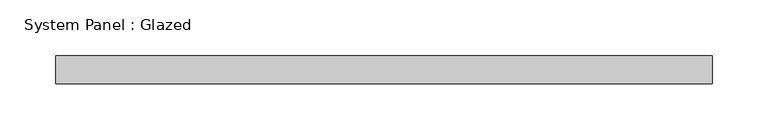
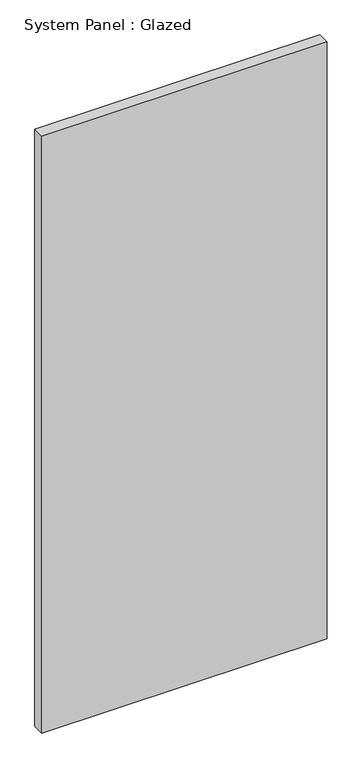
"""IFC4 building model written with IfcOpenShell, lengths in millimetres: plate geometry, System Panel : Glazed."""

from ifc_helpers import new_model, si_unit, origin, origin_with_axes, place, context, project, spatial, polyline, outline, extrude, source, transform, mapped, element, save


def system_panel_glazed_f1c06e49(model_context):
    return source(origin(), model_context, "Body", "SweptSolid", [
        extrude(outline(polyline([(295.275, 19.05), (-295.275, 19.05), (-295.275, 44.45), (295.275, 44.45), (295.275, 19.05)])), origin_with_axes(), (0.0, 0.0, 1.0), 1305.2179754),
    ])


if __name__ == "__main__":
    model = new_model("IFC4")
    model_context = context("Model", 3, world=origin())
    ifc_project = project(units=[si_unit("LENGTHUNIT", "METRE", prefix="MILLI")], contexts=[model_context])
    site = spatial("IfcSite", under=ifc_project)
    building = spatial("IfcBuilding", under=site)
    placement = place(None, origin())
    system_panel_glazed_shape = system_panel_glazed_f1c06e49(model_context)
    element("IfcPlate", 1, ObjectType="System Panel : Glazed", at=placement, inside=building, context=model_context, shape_type="MappedRepresentation", body=[
        mapped(system_panel_glazed_shape, transform((0.0, 0.0, 0.0), x_axis=(1.0, 0.0, 0.0), y_axis=(0.0, 1.0, 0.0), z_axis=(0.0, 0.0, 1.0))),
    ])
    save(model, "model.ifc")

# Revit data of these elements
# Type "System Panel : Glazed"
#   Construction Type Id = "GSP4R"
#   Analytic Construction = "1/8 in Pilkington single glazing"
#   Visual Light Transmittance = 0.9
#   Solar Heat Gain Coefficient = 0.86
#   Heat Transfer Coefficient (U) = 1.18115 BTU/(h·ft²·°F)
#   Define Thermal Properties by = 1
# Element 1 (IfcPlate, "System Panel : Glazed")
#   Materials on its faces: "Glass"
# Materials
#   "Glass": class "Glass", colour RGB 0 128 192, transparency 0.75, Description = "Soda Lime Glass", Cost = 0
